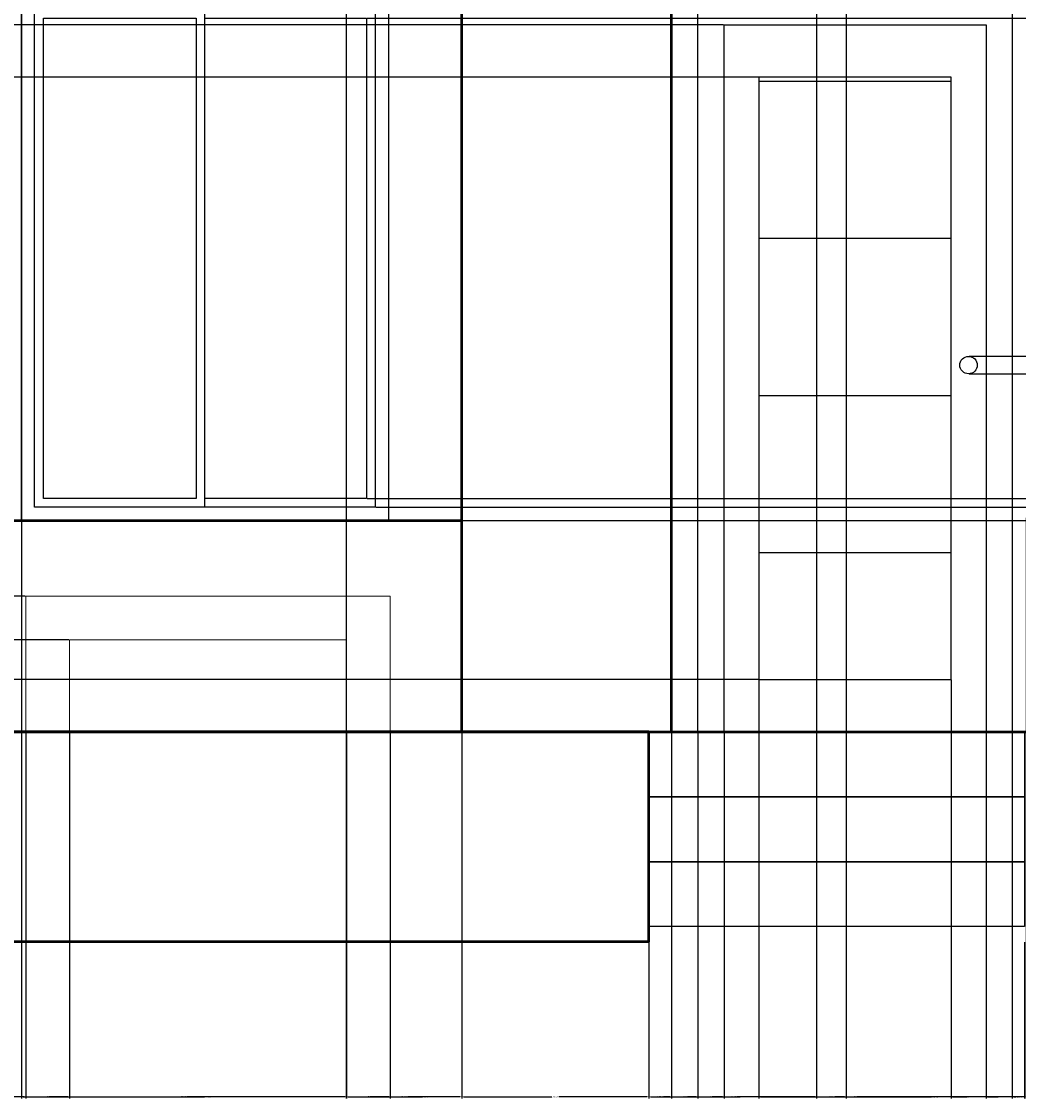
# Model space of a CAD drawing. Units: inches. Extents: x 27 to 409, y -26 to 294.
# Tile 2 of 7: x 116 to 230, y -26 to 97. Entities that reach past the tile are written whole.
import ezdxf

# ---------------------------------------------------------------- set-up
doc = ezdxf.new("R2010")
doc.units = ezdxf.units.IN
doc.header["$MEASUREMENT"] = 0
for name, color, linetype, lineweight in [('A-ANNO-DIMS', 2, 'Continuous', 18), ('A-DOOR', 3, 'Continuous', 25), ('A-ELEV', 8, 'Continuous', 18), ('A-FLOR-STRS', 2, 'Continuous', 25), ('A-GLAZ', 4, 'Continuous', 25), ('A-WALL', 7, 'Continuous', 50)]:
    doc.layers.add(name, color=color, linetype=linetype, lineweight=lineweight)
doc.styles.get("Standard").update_dxf_attribs({"font": 'arial.ttf'})
doc.dimstyles.get("Standard").update_dxf_attribs({"dimtxt": 0.18, "dimasz": 0.18, "dimexe": 0.18, "dimexo": 0.0625, "dimgap": 0.09, "dimtad": 0, "dimtih": 1, "dimtoh": 1, "dimdec": 4, "dimzin": 0, "dimdsep": 46, "dimtxsty": 'Standard', "dimcen": 0.09, "dimadec": 0, "dimazin": 0, "dimtfac": 1, "dimtdec": 4, "dimtofl": 0, "dimtmove": 0, "dimatfit": 3, "dimfxl": 1, "dimtolj": 1, "dimtzin": 0, "dimarcsym": 0})

# ---------------------------------------------------------------- blocks, each defined once
blk = doc.blocks.new('*U2')
for p, q in [((1.5, 1.5), (1.5, 58.5)), ((1.5, 58.5), (21, 58.5)), ((21, 1.5), (21, 58.5)), ((21, 58.5), (40.5, 58.5)), ((40.5, 58.5), (40.5, 1.5)), ((21, 1.5), (1.5, 1.5)), ((40.5, 1.5), (21, 1.5))]:
    blk.add_line(p, q)
blk.add_lwpolyline([(0, 0), (0, 60), (42, 60), (42, 0)], close=True)
for points in [[(20, 57.5), (20, 2.5), (2.5, 2.5), (2.5, 57.5), (20, 57.5)], [(21, 57.5), (39.5, 57.5), (39.5, 2.5), (21, 2.5)]]:
    blk.add_lwpolyline(points)
blk = doc.blocks.new('*U5')
blk.add_lwpolyline([(3.12, 0.01), (0.12, 0.01), (0.12, 84.01), (36.12, 84.01), (36.12, 0.01), (33.12, 0.01)])
for points in [[(33.12, 80.99), (33.12, 0.01), (3.12, 0.01), (3.12, 80.99)], [(29.12, 6.01), (29.12, 74.99), (7.12, 74.99), (7.12, 6.01)]]:
    blk.add_lwpolyline(points, close=True)
blk.add_circle((31.12, 42.01), 1)
blk = doc.blocks.new('*D15')
at = {"layer": 'A-ANNO-DIMS', "color": 0, "lineweight": -2, "transparency": 16777216}
for p, q in [((152.83, 275.59), (152.83, -26.5)), ((115.67, 115.93), (115.67, -26.5)), ((115.85, -26.32), (133.86, -26.32)), ((152.65, -26.32), (134.64, -26.32))]:
    blk.add_line(p, q, dxfattribs=at)
at = {"layer": 'A-ANNO-DIMS', "color": 0, "transparency": 16777216}
for points in [[(115.85, -26.29), (115.85, -26.35), (115.67, -26.32)], [(152.65, -26.29), (152.65, -26.35), (152.83, -26.32)]]:
    blk.add_solid(points, dxfattribs=at)
at = {"layer": 'Defpoints', "color": 0, "transparency": 16777216}
for p in [(152.83, 275.65), (115.67, 116), (152.83, -26.32)]:
    blk.add_point(p, dxfattribs=at)
at = {"layer": 'A-ANNO-DIMS', "color": 0, "transparency": 16777216, "insert": (134.25, -26.32), "char_height": 0.18, "attachment_point": 5}
blk.add_mtext('\\A1;37.17', dxfattribs=at)
blk = doc.blocks.new('*D16')
at = {"layer": 'A-ANNO-DIMS', "color": 0, "lineweight": -2, "transparency": 16777216}
for p, q in [((152.83, 275.59), (152.83, -26.5)), ((166.08, 180.52), (166.08, -26.5)), ((153.01, -26.32), (159, -26.32)), ((165.9, -26.32), (159.91, -26.32))]:
    blk.add_line(p, q, dxfattribs=at)
at = {"layer": 'A-ANNO-DIMS', "color": 0, "transparency": 16777216}
for points in [[(153.01, -26.29), (153.01, -26.35), (152.83, -26.32)], [(165.9, -26.29), (165.9, -26.35), (166.08, -26.32)]]:
    blk.add_solid(points, dxfattribs=at)
at = {"layer": 'Defpoints', "color": 0, "transparency": 16777216}
for p in [(152.83, 275.65), (166.08, 180.59), (166.08, -26.32)]:
    blk.add_point(p, dxfattribs=at)
at = {"layer": 'A-ANNO-DIMS', "color": 0, "transparency": 16777216, "insert": (159.45, -26.32), "char_height": 0.18, "attachment_point": 5}
blk.add_mtext('\\A1;13.242', dxfattribs=at)
blk = doc.blocks.new('*D17')
at = {"layer": 'A-ANNO-DIMS', "color": 0, "lineweight": -2, "transparency": 16777216}
for p, q in [((166.08, 180.52), (166.08, -26.5)), ((187.49, -8.58), (187.49, -26.5)), ((166.26, -26.32), (176.39, -26.32)), ((187.31, -26.32), (177.18, -26.32))]:
    blk.add_line(p, q, dxfattribs=at)
at = {"layer": 'A-ANNO-DIMS', "color": 0, "transparency": 16777216}
for points in [[(166.26, -26.29), (166.26, -26.35), (166.08, -26.32)], [(187.31, -26.29), (187.31, -26.35), (187.49, -26.32)]]:
    blk.add_solid(points, dxfattribs=at)
at = {"layer": 'Defpoints', "color": 0, "transparency": 16777216}
for p in [(166.08, 180.59), (187.49, -8.52), (187.49, -26.32)]:
    blk.add_point(p, dxfattribs=at)
at = {"layer": 'A-ANNO-DIMS', "color": 0, "transparency": 16777216, "insert": (176.78, -26.32), "char_height": 0.18, "attachment_point": 5}
blk.add_mtext('\\A1;21.42', dxfattribs=at)
blk = doc.blocks.new('*D18')
at = {"layer": 'A-ANNO-DIMS', "color": 0, "lineweight": -2, "transparency": 16777216}
for p, q in [((206.7, 130.47), (206.7, -26.5)), ((187.49, -8.58), (187.49, -26.5)), ((187.67, -26.32), (196.64, -26.32)), ((206.52, -26.32), (197.55, -26.32))]:
    blk.add_line(p, q, dxfattribs=at)
at = {"layer": 'A-ANNO-DIMS', "color": 0, "transparency": 16777216}
for points in [[(187.67, -26.29), (187.67, -26.35), (187.49, -26.32)], [(206.52, -26.29), (206.52, -26.35), (206.7, -26.32)]]:
    blk.add_solid(points, dxfattribs=at)
at = {"layer": 'Defpoints', "color": 0, "transparency": 16777216}
for p in [(206.7, 130.53), (187.49, -8.52), (206.7, -26.32)]:
    blk.add_point(p, dxfattribs=at)
at = {"layer": 'A-ANNO-DIMS', "color": 0, "transparency": 16777216, "insert": (197.09, -26.32), "char_height": 0.18, "attachment_point": 5}
blk.add_mtext('\\A1;19.203', dxfattribs=at)
blk = doc.blocks.new('*D19')
at = {"layer": 'A-ANNO-DIMS', "color": 0, "lineweight": -2, "transparency": 16777216}
for p, q in [((210.09, 143.71), (210.09, -26.5)), ((206.7, 130.47), (206.7, -26.5)), ((206.88, -26.32), (208, -26.32)), ((209.91, -26.32), (208.79, -26.32))]:
    blk.add_line(p, q, dxfattribs=at)
at = {"layer": 'A-ANNO-DIMS', "color": 0, "transparency": 16777216}
for points in [[(206.88, -26.29), (206.88, -26.35), (206.7, -26.32)], [(209.91, -26.29), (209.91, -26.35), (210.09, -26.32)]]:
    blk.add_solid(points, dxfattribs=at)
at = {"layer": 'Defpoints', "color": 0, "transparency": 16777216}
for p in [(210.09, 143.77), (206.7, 130.53), (210.09, -26.32)]:
    blk.add_point(p, dxfattribs=at)
at = {"layer": 'A-ANNO-DIMS', "color": 0, "transparency": 16777216, "insert": (208.39, -26.32), "char_height": 0.18, "attachment_point": 5}
blk.add_mtext('\\A1;3.394', dxfattribs=at)
blk = doc.blocks.new('*D20')
at = {"layer": 'A-ANNO-DIMS', "color": 0, "lineweight": -2, "transparency": 16777216}
for p, q in [((210.09, 143.71), (210.09, -26.5)), ((230.52, -8.58), (230.52, -26.5)), ((210.27, -26.32), (219.84, -26.32)), ((230.34, -26.32), (220.77, -26.32))]:
    blk.add_line(p, q, dxfattribs=at)
at = {"layer": 'A-ANNO-DIMS', "color": 0, "transparency": 16777216}
for points in [[(210.27, -26.29), (210.27, -26.35), (210.09, -26.32)], [(230.34, -26.29), (230.34, -26.35), (230.52, -26.32)]]:
    blk.add_solid(points, dxfattribs=at)
at = {"layer": 'Defpoints', "color": 0, "transparency": 16777216}
for p in [(210.09, 143.77), (230.52, -8.52), (230.52, -26.32)]:
    blk.add_point(p, dxfattribs=at)
at = {"layer": 'A-ANNO-DIMS', "color": 0, "transparency": 16777216, "insert": (220.31, -26.32), "char_height": 0.18, "attachment_point": 5}
blk.add_mtext('\\A1;20.435', dxfattribs=at)
blk = doc.blocks.new('*D53')
at = {"layer": 'A-ANNO-DIMS', "color": 0, "lineweight": -2, "transparency": 16777216}
for p, q in [((187.49, 15.42), (187.49, -26.5)), ((190.08, 15.42), (190.08, -26.5)), ((187.67, -26.32), (188.39, -26.32)), ((189.9, -26.32), (189.18, -26.32))]:
    blk.add_line(p, q, dxfattribs=at)
at = {"layer": 'A-ANNO-DIMS', "color": 0, "transparency": 16777216}
for points in [[(187.67, -26.29), (187.67, -26.35), (187.49, -26.32)], [(189.9, -26.29), (189.9, -26.35), (190.08, -26.32)]]:
    blk.add_solid(points, dxfattribs=at)
at = {"layer": 'Defpoints', "color": 0, "transparency": 16777216}
for p in [(187.49, 15.48), (190.08, 15.48), (190.08, -26.32)]:
    blk.add_point(p, dxfattribs=at)
at = {"layer": 'A-ANNO-DIMS', "color": 0, "transparency": 16777216, "insert": (188.78, -26.32), "char_height": 0.18, "attachment_point": 5}
blk.add_mtext('\\A1;2.582', dxfattribs=at)
blk = doc.blocks.new('*D54')
at = {"layer": 'A-ANNO-DIMS', "color": 0, "lineweight": -2, "transparency": 16777216}
for p, q in [((190.08, 15.42), (190.08, -26.5)), ((193.1, 15.43), (193.1, -26.5)), ((190.26, -26.32), (191.27, -26.32)), ((192.92, -26.32), (191.91, -26.32))]:
    blk.add_line(p, q, dxfattribs=at)
at = {"layer": 'A-ANNO-DIMS', "color": 0, "transparency": 16777216}
for points in [[(190.26, -26.29), (190.26, -26.35), (190.08, -26.32)], [(192.92, -26.29), (192.92, -26.35), (193.1, -26.32)]]:
    blk.add_solid(points, dxfattribs=at)
at = {"layer": 'Defpoints', "color": 0, "transparency": 16777216}
for p in [(190.08, 15.48), (193.1, 15.5), (193.1, -26.32)]:
    blk.add_point(p, dxfattribs=at)
at = {"layer": 'A-ANNO-DIMS', "color": 0, "transparency": 16777216, "insert": (191.59, -26.32), "char_height": 0.18, "attachment_point": 5}
blk.add_mtext('\\A1;3.03', dxfattribs=at)
blk = doc.blocks.new('*D55')
at = {"layer": 'A-ANNO-DIMS', "color": 0, "lineweight": -2, "transparency": 16777216}
for p, q in [((193.1, 15.43), (193.1, -26.5)), ((196.1, 15.43), (196.1, -26.5)), ((193.28, -26.32), (194.45, -26.32)), ((195.92, -26.32), (194.75, -26.32))]:
    blk.add_line(p, q, dxfattribs=at)
at = {"layer": 'A-ANNO-DIMS', "color": 0, "transparency": 16777216}
for points in [[(193.28, -26.29), (193.28, -26.35), (193.1, -26.32)], [(195.92, -26.29), (195.92, -26.35), (196.1, -26.32)]]:
    blk.add_solid(points, dxfattribs=at)
at = {"layer": 'Defpoints', "color": 0, "transparency": 16777216}
for p in [(193.1, 15.5), (196.1, 15.5), (196.1, -26.32)]:
    blk.add_point(p, dxfattribs=at)
at = {"layer": 'A-ANNO-DIMS', "color": 0, "transparency": 16777216, "insert": (194.6, -26.32), "char_height": 0.18, "attachment_point": 5}
blk.add_mtext('\\A1;3', dxfattribs=at)
blk = doc.blocks.new('*D56')
at = {"layer": 'A-ANNO-DIMS', "color": 0, "lineweight": -2, "transparency": 16777216}
for p, q in [((200.1, 21.43), (200.1, -26.5)), ((196.1, 15.43), (196.1, -26.5)), ((196.28, -26.32), (197.95, -26.32)), ((199.92, -26.32), (198.26, -26.32))]:
    blk.add_line(p, q, dxfattribs=at)
at = {"layer": 'A-ANNO-DIMS', "color": 0, "transparency": 16777216}
for points in [[(196.28, -26.29), (196.28, -26.35), (196.1, -26.32)], [(199.92, -26.29), (199.92, -26.35), (200.1, -26.32)]]:
    blk.add_solid(points, dxfattribs=at)
at = {"layer": 'Defpoints', "color": 0, "transparency": 16777216}
for p in [(200.1, 21.5), (196.1, 15.5), (200.1, -26.32)]:
    blk.add_point(p, dxfattribs=at)
at = {"layer": 'A-ANNO-DIMS', "color": 0, "transparency": 16777216, "insert": (198.1, -26.32), "char_height": 0.18, "attachment_point": 5}
blk.add_mtext('\\A1;4', dxfattribs=at)
blk = doc.blocks.new('*D57')
at = {"layer": 'A-ANNO-DIMS', "color": 0, "lineweight": -2, "transparency": 16777216}
for p, q in [((200.1, 21.43), (200.1, -26.5)), ((222.1, 21.43), (222.1, -26.5)), ((200.28, -26.32), (210.88, -26.32)), ((221.92, -26.32), (211.32, -26.32))]:
    blk.add_line(p, q, dxfattribs=at)
at = {"layer": 'A-ANNO-DIMS', "color": 0, "transparency": 16777216}
for points in [[(200.28, -26.29), (200.28, -26.35), (200.1, -26.32)], [(221.92, -26.29), (221.92, -26.35), (222.1, -26.32)]]:
    blk.add_solid(points, dxfattribs=at)
at = {"layer": 'Defpoints', "color": 0, "transparency": 16777216}
for p in [(200.1, 21.5), (222.1, 21.5), (222.1, -26.32)]:
    blk.add_point(p, dxfattribs=at)
at = {"layer": 'A-ANNO-DIMS', "color": 0, "transparency": 16777216, "insert": (211.1, -26.32), "char_height": 0.18, "attachment_point": 5}
blk.add_mtext('\\A1;22', dxfattribs=at)
blk = doc.blocks.new('*D58')
at = {"layer": 'A-ANNO-DIMS', "color": 0, "lineweight": -2, "transparency": 16777216}
for p, q in [((222.1, 21.43), (222.1, -26.5)), ((226.1, 15.43), (226.1, -26.5)), ((222.28, -26.32), (223.95, -26.32)), ((225.92, -26.32), (224.26, -26.32))]:
    blk.add_line(p, q, dxfattribs=at)
at = {"layer": 'A-ANNO-DIMS', "color": 0, "transparency": 16777216}
for points in [[(222.28, -26.29), (222.28, -26.35), (222.1, -26.32)], [(225.92, -26.29), (225.92, -26.35), (226.1, -26.32)]]:
    blk.add_solid(points, dxfattribs=at)
at = {"layer": 'Defpoints', "color": 0, "transparency": 16777216}
for p in [(222.1, 21.5), (226.1, 15.5), (226.1, -26.32)]:
    blk.add_point(p, dxfattribs=at)
at = {"layer": 'A-ANNO-DIMS', "color": 0, "transparency": 16777216, "insert": (224.1, -26.32), "char_height": 0.18, "attachment_point": 5}
blk.add_mtext('\\A1;4', dxfattribs=at)
blk = doc.blocks.new('*D59')
at = {"layer": 'A-ANNO-DIMS', "color": 0, "lineweight": -2, "transparency": 16777216}
for p, q in [((226.1, 15.43), (226.1, -26.5)), ((229.1, 15.43), (229.1, -26.5)), ((226.28, -26.32), (227.45, -26.32)), ((228.92, -26.32), (227.75, -26.32))]:
    blk.add_line(p, q, dxfattribs=at)
at = {"layer": 'A-ANNO-DIMS', "color": 0, "transparency": 16777216}
for points in [[(226.28, -26.29), (226.28, -26.35), (226.1, -26.32)], [(228.92, -26.29), (228.92, -26.35), (229.1, -26.32)]]:
    blk.add_solid(points, dxfattribs=at)
at = {"layer": 'Defpoints', "color": 0, "transparency": 16777216}
for p in [(226.1, 15.5), (229.1, 15.5), (229.1, -26.32)]:
    blk.add_point(p, dxfattribs=at)
at = {"layer": 'A-ANNO-DIMS', "color": 0, "transparency": 16777216, "insert": (227.6, -26.32), "char_height": 0.18, "attachment_point": 5}
blk.add_mtext('\\A1;3', dxfattribs=at)
blk = doc.blocks.new('*D60')
at = {"layer": 'A-ANNO-DIMS', "color": 0, "lineweight": -2, "transparency": 16777216}
for p, q in [((230.68, 40), (230.68, -26.5)), ((229.1, 15.43), (229.1, -26.5)), ((229.28, -26.32), (229.53, -26.32)), ((230.5, -26.32), (230.26, -26.32))]:
    blk.add_line(p, q, dxfattribs=at)
at = {"layer": 'A-ANNO-DIMS', "color": 0, "transparency": 16777216}
for points in [[(229.28, -26.29), (229.28, -26.35), (229.1, -26.32)], [(230.5, -26.29), (230.5, -26.35), (230.68, -26.32)]]:
    blk.add_solid(points, dxfattribs=at)
at = {"layer": 'Defpoints', "color": 0, "transparency": 16777216}
for p in [(230.68, 40.07), (229.1, 15.5), (230.68, -26.32)]:
    blk.add_point(p, dxfattribs=at)
at = {"layer": 'A-ANNO-DIMS', "color": 0, "transparency": 16777216, "insert": (229.89, -26.32), "char_height": 0.18, "attachment_point": 5}
blk.add_mtext('\\A1;1.581', dxfattribs=at)
blk = doc.blocks.new('*D69')
at = {"layer": 'A-ANNO-DIMS', "color": 0, "lineweight": -2, "transparency": 16777216}
for p, q in [((200.04, 21.5), (27.6, 21.5)), ((27.78, 21.32), (27.78, 18.67)), ((27.78, 15.66), (27.78, 18.31)), ((190.01, 15.48), (27.6, 15.48))]:
    blk.add_line(p, q, dxfattribs=at)
at = {"layer": 'A-ANNO-DIMS', "color": 0, "transparency": 16777216}
for points in [[(27.75, 21.32), (27.81, 21.32), (27.78, 21.5)], [(27.75, 15.66), (27.81, 15.66), (27.78, 15.48)]]:
    blk.add_solid(points, dxfattribs=at)
at = {"layer": 'Defpoints', "color": 0, "transparency": 16777216}
for p in [(27.78, 21.5), (200.1, 21.5), (190.08, 15.48)]:
    blk.add_point(p, dxfattribs=at)
at = {"layer": 'A-ANNO-DIMS', "color": 0, "transparency": 16777216, "insert": (27.78, 18.49), "char_height": 0.18, "attachment_point": 5}
blk.add_mtext('\\A1;6.013', dxfattribs=at)
blk = doc.blocks.new('*D70')
at = {"layer": 'A-ANNO-DIMS', "color": 0, "lineweight": -2, "transparency": 16777216}
for p, q in [((200.04, 90.47), (27.6, 90.47)), ((27.78, 90.29), (27.78, 56.17)), ((27.78, 21.68), (27.78, 55.8)), ((200.04, 21.5), (27.6, 21.5))]:
    blk.add_line(p, q, dxfattribs=at)
at = {"layer": 'A-ANNO-DIMS', "color": 0, "transparency": 16777216}
for points in [[(27.75, 90.29), (27.81, 90.29), (27.78, 90.47)], [(27.75, 21.68), (27.81, 21.68), (27.78, 21.5)]]:
    blk.add_solid(points, dxfattribs=at)
at = {"layer": 'Defpoints', "color": 0, "transparency": 16777216}
for p in [(27.78, 90.47), (200.1, 90.47), (200.1, 21.5)]:
    blk.add_point(p, dxfattribs=at)
at = {"layer": 'A-ANNO-DIMS', "color": 0, "transparency": 16777216, "insert": (27.78, 55.98), "char_height": 0.18, "attachment_point": 5}
blk.add_mtext('\\A1;68.98', dxfattribs=at)
blk = doc.blocks.new('*D71')
at = {"layer": 'A-ANNO-DIMS', "color": 0, "lineweight": -2, "transparency": 16777216}
for p, q in [((196.04, 96.47), (27.6, 96.47)), ((27.78, 96.29), (27.78, 93.65)), ((27.78, 90.65), (27.78, 93.29)), ((200.04, 90.47), (27.6, 90.47))]:
    blk.add_line(p, q, dxfattribs=at)
at = {"layer": 'A-ANNO-DIMS', "color": 0, "transparency": 16777216}
for points in [[(27.75, 96.29), (27.81, 96.29), (27.78, 96.47)], [(27.75, 90.65), (27.81, 90.65), (27.78, 90.47)]]:
    blk.add_solid(points, dxfattribs=at)
at = {"layer": 'Defpoints', "color": 0, "transparency": 16777216}
for p in [(27.78, 96.47), (196.1, 96.47), (200.1, 90.47)]:
    blk.add_point(p, dxfattribs=at)
at = {"layer": 'A-ANNO-DIMS', "color": 0, "transparency": 16777216, "insert": (27.78, 93.47), "char_height": 0.18, "attachment_point": 5}
blk.add_mtext('\\A1;6', dxfattribs=at)
blk = doc.blocks.new('*D72')
at = {"layer": 'A-ANNO-DIMS', "color": 0, "lineweight": -2, "transparency": 16777216}
for p, q in [((190.01, 99.5), (27.6, 99.5)), ((27.78, 99.32), (27.78, 98.17)), ((27.78, 96.65), (27.78, 97.8)), ((196.04, 96.47), (27.6, 96.47))]:
    blk.add_line(p, q, dxfattribs=at)
at = {"layer": 'A-ANNO-DIMS', "color": 0, "transparency": 16777216}
for points in [[(27.75, 99.32), (27.81, 99.32), (27.78, 99.5)], [(27.75, 96.65), (27.81, 96.65), (27.78, 96.47)]]:
    blk.add_solid(points, dxfattribs=at)
at = {"layer": 'Defpoints', "color": 0, "transparency": 16777216}
for p in [(27.78, 99.5), (190.08, 99.5), (196.1, 96.47)]:
    blk.add_point(p, dxfattribs=at)
at = {"layer": 'A-ANNO-DIMS', "color": 0, "transparency": 16777216, "insert": (27.78, 97.98), "char_height": 0.18, "attachment_point": 5}
blk.add_mtext('\\A1;3.023', dxfattribs=at)
blk = doc.blocks.new('*D74')
at = {"layer": 'A-ANNO-DIMS', "color": 0, "lineweight": -2, "transparency": 16777216}
for p, q in [((224.17, 56.5), (408.69, 56.5)), ((408.51, 56.32), (408.51, 36.18)), ((408.51, 15.68), (408.51, 35.81)), ((226.17, 15.5), (408.69, 15.5))]:
    blk.add_line(p, q, dxfattribs=at)
at = {"layer": 'A-ANNO-DIMS', "color": 0, "transparency": 16777216}
for points in [[(408.48, 56.32), (408.54, 56.32), (408.51, 56.5)], [(408.48, 15.68), (408.54, 15.68), (408.51, 15.5)]]:
    blk.add_solid(points, dxfattribs=at)
at = {"layer": 'Defpoints', "color": 0, "transparency": 16777216}
for p in [(224.1, 56.5), (408.51, 56.5), (226.1, 15.5)]:
    blk.add_point(p, dxfattribs=at)
at = {"layer": 'A-ANNO-DIMS', "color": 0, "transparency": 16777216, "insert": (408.51, 36), "char_height": 0.18, "attachment_point": 5}
blk.add_mtext('\\A1;41', dxfattribs=at)
blk = doc.blocks.new('*D75')
at = {"layer": 'A-ANNO-DIMS', "color": 0, "lineweight": -2, "transparency": 16777216}
for p, q in [((224.17, 58.5), (408.69, 58.5)), ((408.51, 58.32), (408.51, 57.68)), ((408.51, 56.68), (408.51, 57.31)), ((224.17, 56.5), (408.69, 56.5))]:
    blk.add_line(p, q, dxfattribs=at)
at = {"layer": 'A-ANNO-DIMS', "color": 0, "transparency": 16777216}
for points in [[(408.48, 58.32), (408.54, 58.32), (408.51, 58.5)], [(408.48, 56.68), (408.54, 56.68), (408.51, 56.5)]]:
    blk.add_solid(points, dxfattribs=at)
at = {"layer": 'Defpoints', "color": 0, "transparency": 16777216}
for p in [(224.1, 58.5), (408.51, 58.5), (224.1, 56.5)]:
    blk.add_point(p, dxfattribs=at)
at = {"layer": 'A-ANNO-DIMS', "color": 0, "transparency": 16777216, "insert": (408.51, 57.5), "char_height": 0.18, "attachment_point": 5}
blk.add_mtext('\\A1;2', dxfattribs=at)
blk = doc.blocks.new('*D91')
at = {"layer": 'A-ANNO-DIMS', "color": 0, "lineweight": -2, "transparency": 16777216}
for p, q in [((103.08, 15.42), (103.08, -26.5)), ((116.16, 15.42), (116.16, -26.5)), ((103.26, -26.32), (109.16, -26.32)), ((115.98, -26.32), (110.07, -26.32))]:
    blk.add_line(p, q, dxfattribs=at)
at = {"layer": 'A-ANNO-DIMS', "color": 0, "transparency": 16777216}
for points in [[(103.26, -26.29), (103.26, -26.35), (103.08, -26.32)], [(115.98, -26.29), (115.98, -26.35), (116.16, -26.32)]]:
    blk.add_solid(points, dxfattribs=at)
at = {"layer": 'Defpoints', "color": 0, "transparency": 16777216}
for p in [(103.08, 15.48), (116.16, 15.48), (116.16, -26.32)]:
    blk.add_point(p, dxfattribs=at)
at = {"layer": 'A-ANNO-DIMS', "color": 0, "transparency": 16777216, "insert": (109.62, -26.32), "char_height": 0.18, "attachment_point": 5}
blk.add_mtext('\\A1;13.089', dxfattribs=at)
blk = doc.blocks.new('*D92')
at = {"layer": 'A-ANNO-DIMS', "color": 0, "lineweight": -2, "transparency": 16777216}
for p, q in [((116.16, 15.42), (116.16, -26.5)), ((121.16, 15.42), (121.16, -26.5)), ((116.34, -26.32), (118.51, -26.32)), ((120.98, -26.32), (118.81, -26.32))]:
    blk.add_line(p, q, dxfattribs=at)
at = {"layer": 'A-ANNO-DIMS', "color": 0, "transparency": 16777216}
for points in [[(116.34, -26.29), (116.34, -26.35), (116.16, -26.32)], [(120.98, -26.29), (120.98, -26.35), (121.16, -26.32)]]:
    blk.add_solid(points, dxfattribs=at)
at = {"layer": 'Defpoints', "color": 0, "transparency": 16777216}
for p in [(116.16, 15.48), (121.16, 15.48), (121.16, -26.32)]:
    blk.add_point(p, dxfattribs=at)
at = {"layer": 'A-ANNO-DIMS', "color": 0, "transparency": 16777216, "insert": (118.66, -26.32), "char_height": 0.18, "attachment_point": 5}
blk.add_mtext('\\A1;5', dxfattribs=at)
blk = doc.blocks.new('*D93')
at = {"layer": 'A-ANNO-DIMS', "color": 0, "lineweight": -2, "transparency": 16777216}
for p, q in [((121.16, 15.42), (121.16, -26.5)), ((152.89, 15.42), (152.89, -26.5)), ((121.34, -26.32), (136.63, -26.32)), ((152.71, -26.32), (137.42, -26.32))]:
    blk.add_line(p, q, dxfattribs=at)
at = {"layer": 'A-ANNO-DIMS', "color": 0, "transparency": 16777216}
for points in [[(121.34, -26.29), (121.34, -26.35), (121.16, -26.32)], [(152.71, -26.29), (152.71, -26.35), (152.89, -26.32)]]:
    blk.add_solid(points, dxfattribs=at)
at = {"layer": 'Defpoints', "color": 0, "transparency": 16777216}
for p in [(121.16, 15.48), (152.89, 15.48), (152.89, -26.32)]:
    blk.add_point(p, dxfattribs=at)
at = {"layer": 'A-ANNO-DIMS', "color": 0, "transparency": 16777216, "insert": (137.03, -26.32), "char_height": 0.18, "attachment_point": 5}
blk.add_mtext('\\A1;31.73', dxfattribs=at)
blk = doc.blocks.new('*D94')
at = {"layer": 'A-ANNO-DIMS', "color": 0, "lineweight": -2, "transparency": 16777216}
for p, q in [((152.89, 15.42), (152.89, -26.5)), ((157.89, 15.42), (157.89, -26.5)), ((153.07, -26.32), (155.24, -26.32)), ((157.71, -26.32), (155.54, -26.32))]:
    blk.add_line(p, q, dxfattribs=at)
at = {"layer": 'A-ANNO-DIMS', "color": 0, "transparency": 16777216}
for points in [[(153.07, -26.29), (153.07, -26.35), (152.89, -26.32)], [(157.71, -26.29), (157.71, -26.35), (157.89, -26.32)]]:
    blk.add_solid(points, dxfattribs=at)
at = {"layer": 'Defpoints', "color": 0, "transparency": 16777216}
for p in [(152.89, 15.48), (157.89, 15.48), (157.89, -26.32)]:
    blk.add_point(p, dxfattribs=at)
at = {"layer": 'A-ANNO-DIMS', "color": 0, "transparency": 16777216, "insert": (155.39, -26.32), "char_height": 0.18, "attachment_point": 5}
blk.add_mtext('\\A1;5', dxfattribs=at)
blk = doc.blocks.new('*D95')
at = {"layer": 'A-ANNO-DIMS', "color": 0, "lineweight": -2, "transparency": 16777216}
for p, q in [((157.89, 15.42), (157.89, -26.5)), ((166.08, 15.42), (166.08, -26.5)), ((158.07, -26.32), (161.59, -26.32)), ((165.9, -26.32), (162.38, -26.32))]:
    blk.add_line(p, q, dxfattribs=at)
at = {"layer": 'A-ANNO-DIMS', "color": 0, "transparency": 16777216}
for points in [[(158.07, -26.29), (158.07, -26.35), (157.89, -26.32)], [(165.9, -26.29), (165.9, -26.35), (166.08, -26.32)]]:
    blk.add_solid(points, dxfattribs=at)
at = {"layer": 'Defpoints', "color": 0, "transparency": 16777216}
for p in [(157.89, 15.48), (166.08, 15.48), (166.08, -26.32)]:
    blk.add_point(p, dxfattribs=at)
at = {"layer": 'A-ANNO-DIMS', "color": 0, "transparency": 16777216, "insert": (161.98, -26.32), "char_height": 0.18, "attachment_point": 5}
blk.add_mtext('\\A1;8.183', dxfattribs=at)
blk = doc.blocks.new('*D105')
at = {"layer": 'A-ANNO-DIMS', "color": 0, "lineweight": -2, "transparency": 16777216}
for p, q in [((121.1, 26.04), (27.6, 26.04)), ((27.78, 25.86), (27.78, 20.94)), ((27.78, 15.66), (27.78, 20.58)), ((103.01, 15.48), (27.6, 15.48))]:
    blk.add_line(p, q, dxfattribs=at)
at = {"layer": 'A-ANNO-DIMS', "color": 0, "transparency": 16777216}
for points in [[(27.75, 25.86), (27.81, 25.86), (27.78, 26.04)], [(27.75, 15.66), (27.81, 15.66), (27.78, 15.48)]]:
    blk.add_solid(points, dxfattribs=at)
at = {"layer": 'Defpoints', "color": 0, "transparency": 16777216}
for p in [(27.78, 26.04), (121.16, 26.04), (103.08, 15.48)]:
    blk.add_point(p, dxfattribs=at)
at = {"layer": 'A-ANNO-DIMS', "color": 0, "transparency": 16777216, "insert": (27.78, 20.76), "char_height": 0.18, "attachment_point": 5}
blk.add_mtext('\\A1;10.56', dxfattribs=at)
blk = doc.blocks.new('*D106')
at = {"layer": 'A-ANNO-DIMS', "color": 0, "lineweight": -2, "transparency": 16777216}
for p, q in [((116.1, 31.04), (27.6, 31.04)), ((27.78, 30.86), (27.78, 28.72)), ((27.78, 26.22), (27.78, 28.36)), ((121.1, 26.04), (27.6, 26.04))]:
    blk.add_line(p, q, dxfattribs=at)
at = {"layer": 'A-ANNO-DIMS', "color": 0, "transparency": 16777216}
for points in [[(27.75, 30.86), (27.81, 30.86), (27.78, 31.04)], [(27.75, 26.22), (27.81, 26.22), (27.78, 26.04)]]:
    blk.add_solid(points, dxfattribs=at)
at = {"layer": 'Defpoints', "color": 0, "transparency": 16777216}
for p in [(27.78, 31.04), (116.16, 31.04), (121.16, 26.04)]:
    blk.add_point(p, dxfattribs=at)
at = {"layer": 'A-ANNO-DIMS', "color": 0, "transparency": 16777216, "insert": (27.78, 28.54), "char_height": 0.18, "attachment_point": 5}
blk.add_mtext('\\A1;5', dxfattribs=at)
blk = doc.blocks.new('*D107')
at = {"layer": 'A-ANNO-DIMS', "color": 0, "lineweight": -2, "transparency": 16777216}
for p, q in [((103.01, 39.71), (27.6, 39.71)), ((27.78, 39.53), (27.78, 35.56)), ((27.78, 31.22), (27.78, 35.19)), ((116.1, 31.04), (27.6, 31.04))]:
    blk.add_line(p, q, dxfattribs=at)
at = {"layer": 'A-ANNO-DIMS', "color": 0, "transparency": 16777216}
for points in [[(27.75, 39.53), (27.81, 39.53), (27.78, 39.71)], [(27.75, 31.22), (27.81, 31.22), (27.78, 31.04)]]:
    blk.add_solid(points, dxfattribs=at)
at = {"layer": 'Defpoints', "color": 0, "transparency": 16777216}
for p in [(27.78, 39.71), (103.08, 39.71), (116.16, 31.04)]:
    blk.add_point(p, dxfattribs=at)
at = {"layer": 'A-ANNO-DIMS', "color": 0, "transparency": 16777216, "insert": (27.78, 35.38), "char_height": 0.18, "attachment_point": 5}
blk.add_mtext('\\A1;8.666', dxfattribs=at)
blk = doc.blocks.new('*D108')
at = {"layer": 'A-ANNO-DIMS', "color": 0, "lineweight": -2, "transparency": 16777216}
for p, q in [((156.23, 41.21), (408.69, 41.21)), ((408.51, 41.03), (408.51, 40.64)), ((166.14, 39.71), (408.69, 39.71)), ((408.51, 39.89), (408.51, 40.28))]:
    blk.add_line(p, q, dxfattribs=at)
at = {"layer": 'A-ANNO-DIMS', "color": 0, "transparency": 16777216}
for points in [[(408.48, 41.03), (408.54, 41.03), (408.51, 41.21)], [(408.48, 39.89), (408.54, 39.89), (408.51, 39.71)]]:
    blk.add_solid(points, dxfattribs=at)
at = {"layer": 'Defpoints', "color": 0, "transparency": 16777216}
for p in [(156.17, 41.21), (408.51, 41.21), (166.08, 39.71)]:
    blk.add_point(p, dxfattribs=at)
at = {"layer": 'A-ANNO-DIMS', "color": 0, "transparency": 16777216, "insert": (408.51, 40.46), "char_height": 0.18, "attachment_point": 5}
blk.add_mtext('\\A1;1.5', dxfattribs=at)
blk = doc.blocks.new('*D109')
at = {"layer": 'A-ANNO-DIMS', "color": 0, "lineweight": -2, "transparency": 16777216}
for p, q in [((155.23, 42.21), (408.69, 42.21)), ((408.51, 42.03), (408.51, 41.89)), ((156.23, 41.21), (408.69, 41.21)), ((408.51, 41.39), (408.51, 41.53))]:
    blk.add_line(p, q, dxfattribs=at)
at = {"layer": 'A-ANNO-DIMS', "color": 0, "transparency": 16777216}
for points in [[(408.48, 42.03), (408.54, 42.03), (408.51, 42.21)], [(408.48, 41.39), (408.54, 41.39), (408.51, 41.21)]]:
    blk.add_solid(points, dxfattribs=at)
at = {"layer": 'Defpoints', "color": 0, "transparency": 16777216}
for p in [(155.17, 42.21), (408.51, 42.21), (156.17, 41.21)]:
    blk.add_point(p, dxfattribs=at)
at = {"layer": 'A-ANNO-DIMS', "color": 0, "transparency": 16777216, "insert": (408.51, 41.71), "char_height": 0.18, "attachment_point": 5}
blk.add_mtext('\\A1;1', dxfattribs=at)
blk = doc.blocks.new('*D110')
at = {"layer": 'A-ANNO-DIMS', "color": 0, "lineweight": -2, "transparency": 16777216}
for p, q in [((155.23, 97.21), (408.69, 97.21)), ((408.51, 97.03), (408.51, 69.89)), ((408.51, 42.39), (408.51, 69.53)), ((155.23, 42.21), (408.69, 42.21))]:
    blk.add_line(p, q, dxfattribs=at)
at = {"layer": 'A-ANNO-DIMS', "color": 0, "transparency": 16777216}
for points in [[(408.48, 97.03), (408.54, 97.03), (408.51, 97.21)], [(408.48, 42.39), (408.54, 42.39), (408.51, 42.21)]]:
    blk.add_solid(points, dxfattribs=at)
at = {"layer": 'Defpoints', "color": 0, "transparency": 16777216}
for p in [(155.17, 97.21), (408.51, 97.21), (155.17, 42.21)]:
    blk.add_point(p, dxfattribs=at)
at = {"layer": 'A-ANNO-DIMS', "color": 0, "transparency": 16777216, "insert": (408.51, 69.71), "char_height": 0.18, "attachment_point": 5}
blk.add_mtext('\\A1;55', dxfattribs=at)

msp = doc.modelspace()

# ---------------------------------------------------------------- hatches: boundary and pattern name
at = {"layer": 'A-DOOR'}
h = msp.add_hatch(dxfattribs=at)
h.set_pattern_fill('_USER', color=256, scale=18, pattern_type=0)
h.set_pattern_definition([(0, (0, 0), (0, 18), [])])
h.paths.add_polyline_path([(222.1036, 90.4722), (200.1036, 90.4722), (200.1036, 21.4952), (222.1036, 21.4952)])

# ---------------------------------------------------------------- linework, layer by layer
at = {"layer": 'A-ELEV'}
msp.add_line((116.1637, 15.4825), (157.8917, 15.4825), dxfattribs=at)
for points in [[(157.8917, 15.4825), (157.8917, 31.043), (116.1637, 31.043), (116.1637, 15.4825)], [(152.8917, 15.4825), (152.8917, 26.043), (121.1637, 26.043), (121.1637, 15.4825)]]:
    msp.add_lwpolyline(points, dxfattribs=at)
at = {"layer": 'A-FLOR-STRS'}
for points in [[(187.493, 15.4825), (230.5245, 15.4825), (230.5245, 8.0492), (187.493, 8.0492)], [(187.493, 8.0492), (230.5245, 8.0492), (230.5245, 0.6158), (187.493, 0.6158)], [(187.493, 0.6158), (230.5245, 0.6158), (230.5245, -6.8175), (187.493, -6.8175)]]:
    msp.add_lwpolyline(points, close=True, dxfattribs=at)
at = {"layer": 'A-WALL'}
for p, q in [((166.0751, 15.4825), (166.0751, 99.4952)), ((190.0751, 15.4825), (190.0751, 99.4952)), ((103.0751, 39.7093), (166.0751, 39.7093)), ((94.0751, 15.4825), (334.0751, 15.4825))]:
    msp.add_line(p, q, dxfattribs=at)
msp.add_lwpolyline([(187.493, 15.4825), (81.814, 15.4825), (81.814, -8.5175), (187.493, -8.5175)], close=True, dxfattribs=at)

# ---------------------------------------------------------------- block references
at = {"layer": 'A-DOOR'}
msp.add_blockref('*U5', (192.9798, 15.4825), dxfattribs=at)
at = {"layer": 'A-GLAZ'}
msp.add_blockref('*U2', (115.6666, 39.7093), dxfattribs=at)

# ---------------------------------------------------------------- dimensions: what is measured, and where the dimension line sits
at = {"layer": 'A-ANNO-DIMS'}
for base, p1, p2, override, picture, middle in [((152.833, -26.3175), (115.6666, 115.9951), (152.833, 275.6517), {"dimdec": 2, "dimlfac": 1, "dimrnd": 0, "dimzin": 0, "dimdsep": 46, "dimlunit": 2}, '*D15', (134.2498, -26.3175)), ((166.0751, -26.3175), (152.833, 275.6517), (166.0751, 180.5852), {"dimdec": 3, "dimlfac": 1, "dimrnd": 0, "dimzin": 0, "dimdsep": 46, "dimlunit": 2}, '*D16', (159.454, -26.3175)), ((187.493, -26.3175), (166.0751, 180.5852), (187.493, -8.5175), {"dimdec": 2, "dimlfac": 1, "dimrnd": 0, "dimzin": 0, "dimdsep": 46, "dimlunit": 2}, '*D17', (176.784, -26.3175)), ((210.0897, -26.3175), (206.6961, 130.5342), (210.0897, 143.7732), {"dimdec": 3, "dimlfac": 1, "dimrnd": 0, "dimzin": 0, "dimdsep": 46, "dimlunit": 2}, '*D19', (208.3929, -26.3175)), ((230.5245, -26.3175), (210.0897, 143.7732), (230.5245, -8.5175), {"dimdec": 3, "dimlfac": 1, "dimrnd": 0, "dimzin": 0, "dimdsep": 46, "dimlunit": 2}, '*D20', (220.3071, -26.3175)), ((206.6961, -26.3175), (187.493, -8.5175), (206.6961, 130.5342), {"dimdec": 3, "dimlfac": 1, "dimrnd": 0, "dimzin": 0, "dimdsep": 46, "dimlunit": 2}, '*D18', (197.0945, -26.3175)), ((230.6845, -26.3175), (229.1036, 15.4952), (230.6845, 40.0674), {"dimdec": 3, "dimlfac": 1, "dimrnd": 0, "dimzin": 0, "dimdsep": 46, "dimlunit": 2}, '*D60', (229.894, -26.3175)), ((200.1036, -26.3175), (196.1036, 15.4952), (200.1036, 21.4952), {"dimdec": 0, "dimlfac": 1, "dimrnd": 0, "dimzin": 0, "dimdsep": 46, "dimlunit": 2}, '*D56', (198.1036, -26.3175)), ((222.1036, -26.3175), (200.1036, 21.4952), (222.1036, 21.4952), {"dimdec": 0, "dimlfac": 1, "dimrnd": 0, "dimzin": 0, "dimdsep": 46, "dimlunit": 2}, '*D57', (211.1036, -26.3175)), ((226.1036, -26.3175), (222.1036, 21.4952), (226.1036, 15.4952), {"dimdec": 0, "dimlfac": 1, "dimrnd": 0, "dimzin": 0, "dimdsep": 46, "dimlunit": 2}, '*D58', (224.1036, -26.3175)), ((116.1637, -26.3175), (103.0751, 15.4825), (116.1637, 15.4825), {"dimdec": 3, "dimlfac": 1, "dimrnd": 0, "dimzin": 0, "dimdsep": 46, "dimlunit": 2}, '*D91', (109.6194, -26.3175)), ((121.1637, -26.3175), (116.1637, 15.4825), (121.1637, 15.4825), {"dimdec": 0, "dimlfac": 1, "dimrnd": 0, "dimzin": 0, "dimdsep": 46, "dimlunit": 2}, '*D92', (118.6637, -26.3175)), ((152.8917, -26.3175), (121.1637, 15.4825), (152.8917, 15.4825), {"dimdec": 2, "dimlfac": 1, "dimrnd": 0, "dimzin": 0, "dimdsep": 46, "dimlunit": 2}, '*D93', (137.0277, -26.3175)), ((157.8917, -26.3175), (152.8917, 15.4825), (157.8917, 15.4825), {"dimdec": 0, "dimlfac": 1, "dimrnd": 0, "dimzin": 0, "dimdsep": 46, "dimlunit": 2}, '*D94', (155.3917, -26.3175)), ((166.0751, -26.3175), (157.8917, 15.4825), (166.0751, 15.4825), {"dimdec": 3, "dimlfac": 1, "dimrnd": 0, "dimzin": 0, "dimdsep": 46, "dimlunit": 2}, '*D95', (161.9834, -26.3175)), ((190.0751, -26.3175), (187.493, 15.4825), (190.0751, 15.4825), {"dimdec": 3, "dimlfac": 1, "dimrnd": 0, "dimzin": 0, "dimdsep": 46, "dimlunit": 2}, '*D53', (188.784, -26.3175)), ((193.1036, -26.3175), (190.0751, 15.4825), (193.1036, 15.4952), {"dimdec": 2, "dimlfac": 1, "dimrnd": 0, "dimzin": 0, "dimdsep": 46, "dimlunit": 2}, '*D54', (191.5893, -26.3175)), ((196.1036, -26.3175), (193.1036, 15.4952), (196.1036, 15.4952), {"dimdec": 0, "dimlfac": 1, "dimrnd": 0, "dimzin": 0, "dimdsep": 46, "dimlunit": 2}, '*D55', (194.6036, -26.3175)), ((229.1036, -26.3175), (226.1036, 15.4952), (229.1036, 15.4952), {"dimdec": 0, "dimlfac": 1, "dimrnd": 0, "dimzin": 0, "dimdsep": 46, "dimlunit": 2}, '*D59', (227.6036, -26.3175))]:
    dim = msp.add_linear_dim(base=base, p1=p1, p2=p2, dimstyle='Standard', override=override, dxfattribs=at)
    dim.commit()
    dim.dimension.update_dxf_attribs({"geometry": picture, "text_midpoint": middle})
for base, p1, p2, override, picture, middle in [((27.7772, 99.4952), (196.1036, 96.4722), (190.0751, 99.4952), {"dimdec": 3, "dimlfac": 1, "dimrnd": 0, "dimzin": 0, "dimdsep": 46, "dimlunit": 2}, '*D72', (27.7772, 97.9837)), ((27.7772, 96.4722), (200.1036, 90.4722), (196.1036, 96.4722), {"dimdec": 0, "dimlfac": 1, "dimrnd": 0, "dimzin": 0, "dimdsep": 46, "dimlunit": 2}, '*D71', (27.7772, 93.4722)), ((408.5054, 97.2093), (155.1666, 42.2093), (155.1666, 97.2093), {"dimdec": 0, "dimlfac": 1, "dimrnd": 0, "dimzin": 0, "dimdsep": 46, "dimlunit": 2}, '*D110', (408.5054, 69.7093)), ((27.7772, 90.4722), (200.1036, 21.4952), (200.1036, 90.4722), {"dimdec": 2, "dimlfac": 1, "dimrnd": 0, "dimzin": 0, "dimdsep": 46, "dimlunit": 2}, '*D70', (27.7772, 55.9837)), ((408.5054, 58.4952), (224.1036, 56.4952), (224.1036, 58.4952), {"dimdec": 0, "dimlfac": 1, "dimrnd": 0, "dimzin": 0, "dimdsep": 46, "dimlunit": 2}, '*D75', (408.5054, 57.4952)), ((408.5054, 56.4952), (226.1036, 15.4952), (224.1036, 56.4952), {"dimdec": 0, "dimlfac": 1, "dimrnd": 0, "dimzin": 0, "dimdsep": 46, "dimlunit": 2}, '*D74', (408.5054, 35.9952)), ((408.5054, 42.2093), (156.1666, 41.2093), (155.1666, 42.2093), {"dimdec": 0, "dimlfac": 1, "dimrnd": 0, "dimzin": 0, "dimdsep": 46, "dimlunit": 2}, '*D109', (408.5054, 41.7093)), ((408.5054, 41.2093), (166.0751, 39.7093), (156.1666, 41.2093), {"dimdec": 1, "dimlfac": 1, "dimrnd": 0, "dimzin": 0, "dimdsep": 46, "dimlunit": 2}, '*D108', (408.5054, 40.4593)), ((27.7772, 39.7093), (116.1637, 31.043), (103.0751, 39.7093), {"dimdec": 3, "dimlfac": 1, "dimrnd": 0, "dimzin": 0, "dimdsep": 46, "dimlunit": 2}, '*D107', (27.7772, 35.3761)), ((27.7772, 31.043), (121.1637, 26.043), (116.1637, 31.043), {"dimdec": 0, "dimlfac": 1, "dimrnd": 0, "dimzin": 0, "dimdsep": 46, "dimlunit": 2}, '*D106', (27.7772, 28.543)), ((27.7772, 26.043), (103.0751, 15.4825), (121.1637, 26.043), {"dimdec": 2, "dimlfac": 1, "dimrnd": 0, "dimzin": 0, "dimdsep": 46, "dimlunit": 2}, '*D105', (27.7772, 20.7627)), ((27.7772, 21.4952), (190.0751, 15.4825), (200.1036, 21.4952), {"dimdec": 3, "dimlfac": 1, "dimrnd": 0, "dimzin": 0, "dimdsep": 46, "dimlunit": 2}, '*D69', (27.7772, 18.4888))]:
    dim = msp.add_linear_dim(base=base, p1=p1, p2=p2, angle=90, dimstyle='Standard', override=override, dxfattribs=at)
    dim.commit()
    dim.dimension.update_dxf_attribs({"geometry": picture, "text_midpoint": middle})

doc.saveas('drawing.dxf')
